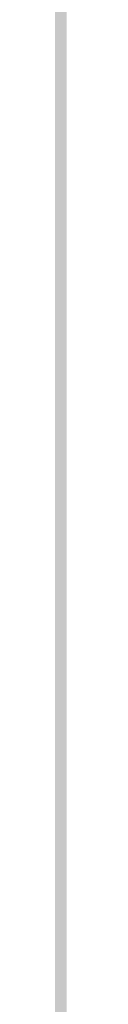
# Model space of a CAD drawing. Units: inches. Extents: x 2083 to 3317, y 1141 to 2115.
# Tile 209 of 256: x 3126.956 to 3126.958, y 1264.131 to 1265.165. Entities that reach past the tile are written whole.
import ezdxf

# ---------------------------------------------------------------- set-up
doc = ezdxf.new("R2010")
doc.units = ezdxf.units.IN
doc.layers.add('A-ANNO-DIMS', color=2, linetype='Continuous', lineweight=18)
doc.layers.add('A-WALL-PATT', color=251, linetype='Continuous', lineweight=13, true_color=0x636466)
doc.styles.get("Standard").update_dxf_attribs({"font": 'arial.ttf'})
doc.dimstyles.new('ISO-25', dxfattribs={"dimtxt": 12, "dimasz": 12, "dimexe": 1.25, "dimexo": 0.625, "dimtad": 1, "dimlunit": 3, "dimtxsty": 'Standard', "dimcen": 2.5, "dimadec": 0, "dimazin": 0, "dimtfac": 1, "dimtmove": 0, "dimatfit": 3, "dimfxl": 1, "dimarcsym": 0})

# ---------------------------------------------------------------- blocks, each defined once
blk = doc.blocks.new('*D26')
at = {"layer": 'A-ANNO-DIMS', "color": 0, "lineweight": -2, "transparency": 16777216}
for p, q in [((3088.9858, 1274.9151), (3088.9858, 1270.952)), ((3111.24, 1274.9151), (3111.24, 1270.952)), ((3076.9858, 1272.202), (2840.2624, 1272.202)), ((3111.24, 1272.202), (3088.9858, 1272.202)), ((3123.24, 1272.202), (3135.24, 1272.202))]:
    blk.add_line(p, q, dxfattribs=at)
at = {"layer": 'A-ANNO-DIMS', "color": 0, "transparency": 16777216}
for points in [[(3076.9858, 1274.202), (3076.9858, 1270.202), (3088.9858, 1272.202)], [(3123.24, 1274.202), (3123.24, 1270.202), (3111.24, 1272.202)]]:
    blk.add_solid(points, dxfattribs=at)
at = {"layer": 'Defpoints', "color": 0, "transparency": 16777216}
for p in [(3088.9858, 1275.5401), (3111.24, 1275.5401), (3088.9858, 1272.202)]:
    blk.add_point(p, dxfattribs=at)
at = {"layer": 'A-ANNO-DIMS', "color": 0, "transparency": 16777216, "insert": (2952.6241, 1279.0316), "char_height": 12, "attachment_point": 5}
blk.add_mtext('NIGHTSTAND 1\'-10 1/2" TYP.', dxfattribs=at)
blk = doc.blocks.new('*D27')
at = {"layer": 'A-ANNO-DIMS', "color": 0, "lineweight": -2, "transparency": 16777216}
for p, q in [((3114.5782, 1309.7943), (3114.5782, 1321.7943)), ((3111.865, 1297.7943), (3115.8282, 1297.7943)), ((3114.5782, 1297.7943), (3114.5782, 1275.5401)), ((3111.865, 1275.5401), (3115.8282, 1275.5401)), ((3114.5782, 1263.5401), (3114.5782, 1140.9886))]:
    blk.add_line(p, q, dxfattribs=at)
at = {"layer": 'A-ANNO-DIMS', "color": 0, "transparency": 16777216}
for points in [[(3112.5782, 1309.7943), (3116.5782, 1309.7943), (3114.5782, 1297.7943)], [(3112.5782, 1263.5401), (3116.5782, 1263.5401), (3114.5782, 1275.5401)]]:
    blk.add_solid(points, dxfattribs=at)
at = {"layer": 'Defpoints', "color": 0, "transparency": 16777216}
for p in [(3111.24, 1297.7943), (3111.24, 1275.5401), (3114.5782, 1275.5401)]:
    blk.add_point(p, dxfattribs=at)
at = {"layer": 'A-ANNO-DIMS', "color": 0, "transparency": 16777216, "insert": (3107.7485, 1196.2643), "char_height": 12, "attachment_point": 5, "rotation": 90}
blk.add_mtext('1\'-10 1/2" TYP.', dxfattribs=at)

msp = doc.modelspace()

# ---------------------------------------------------------------- hatches: boundary and pattern name
at = {"layer": 'A-WALL-PATT'}
h = msp.add_hatch(color=256, dxfattribs=at)
h.dxf.hatch_style = 1
h.paths.add_polyline_path([(3126.9598, 2020.7614), (2748.9598, 2020.7614), (2604.9598, 2020.7614), (2226.9598, 2020.7614), (2226.9598, 1702.7614), (2466.9598, 1702.7614), (2466.9598, 1582.7614), (2418.9598, 1582.7614), (2418.9598, 1477.7614), (2226.9598, 1477.7614), (2226.9598, 1263.2614), (2544.9598, 1263.2614), (2544.9598, 1411.7614), (2604.9598, 1411.7614), (2685.9598, 1411.7614), (2685.9598, 1420.7614), (2604.9598, 1420.7614), (2604.9598, 1573.7614), (2604.9598, 1702.7614), (2604.9598, 2011.7614), (2748.9598, 2011.7614), (2748.9598, 1702.7614), (2862.9598, 1702.7614), (2862.9598, 1621.7614), (2871.9598, 1621.7614), (2871.9598, 1702.7614), (2883.9598, 1702.7614), (2883.9598, 1706.9395, -0.026459), (2883.9598, 1711.7614), (2757.9598, 1711.7614), (2757.9598, 1807.7614), (2787.9598, 1807.7614), (2787.9598, 1812.2614), (2757.9598, 1812.2614), (2757.9598, 2011.7614), (2877.9598, 2011.7614), (2877.9598, 1812.2614), (2847.9598, 1812.2614), (2847.9598, 1807.7614), (2889.8357, 1807.7614), (2889.8357, 1812.2614), (2882.4598, 1812.2614), (2882.4598, 2011.7614), (3117.9598, 2011.7614), (3117.9598, 1812.2614), (2937.8357, 1812.2614), (2937.8357, 1807.7614), (2995.7098, 1807.7614), (2995.7098, 1796.1177), (3000.2098, 1796.1177), (3000.2098, 1807.7614), (3117.9598, 1807.7614), (3117.9598, 1711.7614), (3000.2098, 1711.7614), (3000.2098, 1760.1177), (2998.5727, 1760.1177, -0.020711), (2995.7098, 1760.1177), (2995.7098, 1711.7614), (2931.9598, 1711.7614), (2931.9598, 1702.7614), (3126.9598, 1702.7614)])
h.paths.add_polyline_path([(2471.4598, 2011.7614), (2471.4598, 1810.0114), (2462.7169, 1810.0114), (2462.7169, 1805.5114), (2505.9598, 1805.5114), (2505.9598, 1810.0114), (2475.9598, 1810.0114), (2475.9598, 2011.7614), (2595.9598, 2011.7614), (2595.9598, 1810.0114), (2565.9598, 1810.0114), (2565.9598, 1805.5114), (2595.9598, 1805.5114), (2595.9598, 1711.7614), (2235.9598, 1711.7614), (2235.9598, 1805.5114), (2353.7098, 1805.5114), (2353.7098, 1796.0542), (2358.2098, 1796.0542), (2358.2098, 1805.5114), (2414.7169, 1805.5114), (2414.7169, 1810.0114), (2235.9598, 1810.0114), (2235.9598, 2011.7614)], flags=16)
h.paths.add_polyline_path([(2270.2047, 1994.61), (2270.2047, 1970.61), (2246.2047, 1970.61), (2246.2047, 1994.61)], flags=0)
edge = h.paths.add_edge_path(flags=0)
edge.add_ellipse((2332.0274, 1899.7982), major_axis=(-3.043, 3.043), ratio=0.168252, start_angle=-161.3322, end_angle=-156.3071, ccw=False)
edge.add_ellipse((2333.082, 1898.7435), major_axis=(-1.0546, 1.0546), ratio=0.453532, start_angle=-123.371, end_angle=-94.1591)
edge = h.paths.add_edge_path(flags=0)
edge.add_ellipse((2332.0274, 1968.8763), major_axis=(3.043, 3.043), ratio=0.168252, start_angle=18.6678, end_angle=23.6929)
edge.add_spline(control_points=[(2332.9256, 1970.6911), (2332.2268, 1970.3361), (2330.8937, 1969.6589), (2328.4131, 1970.9321), (2327.2039, 1967.7487), (2324.7096, 1969.9556), (2322.5328, 1967.0124), (2320.0128, 1971.2958), (2317.6803, 1968.1578), (2316.0405, 1967.102), (2315.4269, 1966.8096)], knot_values=[0, 0, 0, 0, 2.267059, 4.324559, 6.685584, 8.878641, 11.121502, 14.300359, 17.755284, 19.732645, 19.732645, 19.732645, 19.732645], degree=3, periodic=0)
edge.add_ellipse((2332.0274, 1968.8763), major_axis=(3.043, 3.043), ratio=0.168252, start_angle=18.6678, end_angle=23.6929, ccw=False)
edge.add_ellipse((2333.082, 1969.9309), major_axis=(1.0546, 1.0546), ratio=0.453532, start_angle=56.629, end_angle=85.8409, ccw=False)
edge = h.paths.add_edge_path(flags=0)
edge.add_spline(control_points=[(2296.4283, 1967.9879), (2293.6278, 1965.3363), (2287.7036, 1959.7271), (2299.7439, 1949.9957), (2294.5326, 1935.6685), (2290.5732, 1920.6035), (2293.3941, 1909.9737), (2296.1854, 1904.9665)], knot_values=[0.099185, 0.099185, 0.099185, 0.099185, 0.345301, 0.619822, 0.982653, 1.386093, 1.810555, 1.810555, 1.810555, 1.810555], degree=3, periodic=0)
edge.add_spline(control_points=[(2296.1854, 1904.9665), (2297.3836, 1902.6193), (2298.001, 1901.9493), (2298.553, 1901.4682)], knot_values=[0.006246, 0.006246, 0.006246, 0.006246, 0.055476, 0.055476, 0.055476, 0.055476], degree=3, periodic=0)
edge.add_spline(control_points=[(2298.553, 1901.4682), (2297.2586, 1900.9232), (2295.2253, 1900.2321), (2293.0602, 1900.6142), (2292.1014, 1900.7884), (2292.0896, 1900.7906)], knot_values=[0.312835, 0.312835, 0.312835, 0.312835, 0.40178, 0.474987, 0.475903, 0.475903, 0.475903, 0.475903], degree=3, periodic=0)
edge.add_arc((2292.7936, 1904.6641), 3.937, 215.4209, 259.6982, ccw=False)
edge.add_spline(control_points=[(2289.5853, 1902.3823), (2289.4767, 1902.5351), (2289.3685, 1902.688), (2289.2609, 1902.8412)], knot_values=[0.102872, 0.102872, 0.102872, 0.102872, 0.116896, 0.116896, 0.116896, 0.116896], degree=3, periodic=0)
edge.add_spline(control_points=[(2289.2609, 1902.8412), (2288.6866, 1902.5502), (2287.64, 1902.0199), (2285.8813, 1901.874), (2283.853, 1901.5044), (2281.72, 1899.7105), (2278.467, 1899.4929), (2276.1571, 1901.8832), (2272.259, 1899.8041), (2267.7776, 1901.8432), (2262.2439, 1900.184), (2257.4149, 1901.7821), (2254.3184, 1900.7261), (2253.1783, 1900.3373)], knot_values=[0, 0, 0, 0, 1.907977, 3.477176, 5.261074, 7.972851, 11.680248, 13.717921, 16.939592, 22.789562, 27.502503, 33.595215, 37.145618, 37.145618, 37.145618, 37.145618], degree=3, periodic=0)
edge.add_line((2253.1783, 1900.3373), (2250.2442, 1902.8412))
edge.add_line((2250.2442, 1902.8412), (2250.2442, 1965.8333))
edge.add_line((2250.2442, 1965.8333), (2253.1783, 1968.3371))
edge.add_spline(control_points=[(2253.1783, 1968.3371), (2254.3184, 1967.9483), (2257.4149, 1966.8924), (2262.2439, 1968.4904), (2267.7776, 1966.8313), (2271.5267, 1968.5372), (2273.8759, 1967.8283), (2274.2067, 1967.7276)], knot_values=[0, 0, 0, 0, 0.09018, 0.244935, 0.364644, 0.513233, 0.537855, 0.537855, 0.537855, 0.537855], degree=3, periodic=0)
edge.add_arc((2274.3529, 1963.7933), 3.937, 72.0511, 92.1279, ccw=False)
edge.add_arc((2281.2969, 1985.23), 18.5963, 252.05113, 288.56572)
edge.add_arc((2292.3167, 1956.0289), 12.6461, 71.02679, 113.77822, ccw=False)
edge = h.paths.add_edge_path(flags=0)
edge.add_spline(control_points=[(2274.8994, 1951.8562), (2275.0662, 1951.6166), (2275.2327, 1951.3766), (2275.398, 1951.1359)], knot_values=[1.409916, 1.409916, 1.409916, 1.409916, 1.43159, 1.43159, 1.43159, 1.43159], degree=3, periodic=0)
edge.add_spline(control_points=[(2275.398, 1951.1359), (2275.7921, 1950.5619), (2276.1792, 1949.9838), (2276.5455, 1949.3971)], knot_values=[1.358238, 1.358238, 1.358238, 1.358238, 1.409916, 1.409916, 1.409916, 1.409916], degree=3, periodic=0)
edge.add_line((2276.5455, 1949.3971), (2277.4373, 1947.8622))
edge.add_spline(control_points=[(2277.4373, 1947.8622), (2276.3038, 1945.6731), (2274.6397, 1942.4269), (2274.6316, 1938.0939), (2272.7991, 1930.8515), (2274.3564, 1943.897), (2275.9477, 1947.9234), (2276.5455, 1949.3971)], knot_values=[0.005632, 0.005632, 0.005632, 0.005632, 0.186014, 0.266002, 0.357087, 0.59639, 0.739732, 0.739732, 0.739732, 0.739732], degree=3, periodic=0)
edge.add_spline(control_points=[(2276.5455, 1949.3971), (2276.1792, 1949.9838), (2275.7921, 1950.5619), (2275.398, 1951.1359)], knot_values=[1.358238, 1.358238, 1.358238, 1.358238, 1.409916, 1.409916, 1.409916, 1.409916], degree=3, periodic=0)
edge.add_spline(control_points=[(2275.398, 1951.1359), (2274.9425, 1950.0805), (2274.2078, 1948.0253), (2273.9346, 1944.8515), (2272.4685, 1937.6275), (2273.4662, 1945.6965), (2274.7006, 1951.0595), (2274.8994, 1951.8562)], knot_values=[0.104364, 0.104364, 0.104364, 0.104364, 0.189636, 0.269624, 0.36071, 0.600013, 0.644622, 0.644622, 0.644622, 0.644622], degree=3, periodic=0)
h.paths.add_polyline_path([(2269.1675, 1963.1276, -0.357527), (2268.1706, 1960.9764, -0.092561), (2268.1706, 1939.4363, -0.357527), (2269.1675, 1937.2851, -0.357527), (2267.0163, 1938.282, -0.164785), (2254.6856, 1938.282, -0.357527), (2252.5344, 1937.2851, -0.357527), (2253.5313, 1939.4363, -0.092561), (2253.5313, 1960.9764, -0.357527), (2252.5344, 1963.1276, -0.357527), (2254.6856, 1962.1307, -0.164785), (2267.0163, 1962.1307, -0.357527)], flags=0)
h.paths.add_polyline_path([(2248.8741, 1967.8018), (2248.8741, 1957.0277), (2249.4578, 1957.0277), (2249.4578, 1911.6468), (2248.8741, 1911.6468), (2248.8741, 1900.8727), (2246.5119, 1900.8727, 0.197327), (2244.1497, 1902.4569), (2244.1497, 1966.2176, 0.197327), (2246.5119, 1967.8018)], flags=0)
h.paths.add_polyline_path([(2269.1675, 1931.3893, -0.357527), (2268.1706, 1929.2381, -0.092561), (2268.1706, 1907.6981, -0.357527), (2269.1675, 1905.5469, -0.357527), (2267.0163, 1906.5438, -0.164785), (2254.6856, 1906.5438, -0.357527), (2252.5344, 1905.5469, -0.357527), (2253.5313, 1907.6981, -0.092561), (2253.5313, 1929.2381, -0.357527), (2252.5344, 1931.3893, -0.357527), (2254.6856, 1930.3925, -0.164785), (2267.0163, 1930.3925, -0.357527)], flags=0)
edge = h.paths.add_edge_path(flags=0)
edge.add_spline(control_points=[(2276.1969, 1906.7237), (2276.1681, 1909.0289), (2276.114, 1913.3719), (2270.5984, 1924.925), (2273.9052, 1919.0128), (2275.9217, 1916.2621), (2275.4746, 1912.4021), (2277.2579, 1910.3806), (2276.696, 1908.225), (2276.6462, 1906.813), (2276.6178, 1906.0084)], knot_values=[0, 0, 0, 0, 8.61026, 16.221274, 18.843057, 23.804898, 27.440828, 29.356102, 31.203478, 33.650687, 33.650687, 33.650687, 33.650687], degree=3, periodic=0)
edge.add_spline(control_points=[(2276.6178, 1906.0084), (2276.6233, 1905.6241), (2276.4977, 1904.6287), (2275.4418, 1903.8547), (2274.9373, 1903.0804), (2274.8591, 1902.8412)], knot_values=[0.156488, 0.156488, 0.156488, 0.156488, 0.184398, 0.231376, 0.250598, 0.250598, 0.250598, 0.250598], degree=3, periodic=0)
edge.add_line((2274.8591, 1902.8412), (2276.506, 1902.8412))
edge.add_spline(control_points=[(2276.506, 1902.8412), (2276.7883, 1903.0849), (2277.6651, 1904.1252), (2278.2495, 1904.3407), (2277.6539, 1908.5274), (2278.1557, 1906.2278), (2278.1005, 1905.2859), (2278.8467, 1904.069), (2277.8568, 1903.4149), (2277.8742, 1902.991), (2277.9036, 1902.8412)], knot_values=[0.059574, 0.059574, 0.059574, 0.059574, 0.080753, 0.103741, 0.16972, 0.176036, 0.207137, 0.240474, 0.262341, 0.27366, 0.27366, 0.27366, 0.27366], degree=3, periodic=0)
edge.add_line((2277.9036, 1902.8412), (2280.0298, 1902.8412))
edge.add_spline(control_points=[(2280.0298, 1902.8412), (2279.8882, 1903.0884), (2279.4993, 1903.9816), (2280.1523, 1905.9393), (2278.1036, 1909.6578), (2279.7624, 1907.1853), (2280.3279, 1904.8749), (2280.4851, 1903.4896), (2281.4633, 1903.2494), (2281.7583, 1902.9365), (2281.834, 1902.8412)], knot_values=[0.013856, 0.013856, 0.013856, 0.013856, 0.034874, 0.088867, 0.107879, 0.126738, 0.158714, 0.193757, 0.217487, 0.226722, 0.226722, 0.226722, 0.226722], degree=3, periodic=0)
edge.add_spline(control_points=[(2281.834, 1902.8412), (2281.7875, 1902.8267), (2281.647, 1902.783), (2281.3955, 1902.8595), (2281.0881, 1902.9852), (2280.7207, 1903.0609), (2280.3335, 1903.0257), (2280.1248, 1902.8989), (2280.0298, 1902.8412)], knot_values=[0, 0, 0, 0, 0.14413, 0.435517, 0.749276, 1.153046, 1.548371, 1.878348, 1.878348, 1.878348, 1.878348], degree=3, periodic=0)
edge.add_line((2280.0298, 1902.8412), (2277.9036, 1902.8412))
edge.add_spline(control_points=[(2277.9036, 1902.8412), (2277.8929, 1902.7959), (2277.8654, 1902.6796), (2277.6075, 1902.6875), (2277.2741, 1902.8007), (2276.8379, 1902.6198), (2276.5838, 1902.7893), (2276.506, 1902.8412)], knot_values=[0, 0, 0, 0, 0.127189, 0.326199, 0.628009, 1.24357, 1.515331, 1.515331, 1.515331, 1.515331], degree=3, periodic=0)
edge.add_line((2276.506, 1902.8412), (2274.8591, 1902.8412))
edge.add_spline(control_points=[(2274.8591, 1902.8412), (2274.8144, 1902.8986), (2274.7251, 1903.0134), (2274.4935, 1903.119), (2274.2443, 1902.9605), (2273.9371, 1903.1849), (2273.614, 1902.9831), (2273.4083, 1902.883), (2273.3223, 1902.8412)], knot_values=[0, 0, 0, 0, 0.21843, 0.436957, 0.687977, 0.990379, 1.398396, 1.69185, 1.69185, 1.69185, 1.69185], degree=3, periodic=0)
edge.add_spline(control_points=[(2273.3223, 1902.8412), (2273.6167, 1903.4457), (2274.274, 1904.5383), (2276.0272, 1904.5737), (2276.207, 1906.5836), (2276.1969, 1906.7237)], knot_values=[0.012227, 0.012227, 0.012227, 0.012227, 0.059472, 0.106218, 0.134458, 0.134458, 0.134458, 0.134458], degree=3, periodic=0)
h.paths.add_polyline_path([(2270.7761, 1897.7898), (2270.7761, 1873.7898), (2246.7761, 1873.7898), (2246.7761, 1897.7898)], flags=0)
h.paths.add_polyline_path([(2353.7098, 1760.0051), (2353.7098, 1760.0542), (2358.2098, 1760.0542, -0.033729)], flags=0)
h.paths.add_polyline_path([(2321.8191, 1737.5292), (2341.9953, 1737.5292, -0.414214), (2343.2033, 1736.3212), (2343.2033, 1721.0206, -0.414214), (2341.9953, 1719.8127), (2321.8191, 1719.8127, -0.414214), (2320.6112, 1721.0206), (2320.6112, 1736.3212, -0.414214)], flags=0)
h.paths.add_polyline_path([(2324.235, 1736.3212), (2339.5794, 1736.3212, -0.414214), (2341.9953, 1733.9053), (2341.9953, 1725.4497, -0.414214), (2339.5794, 1723.0338), (2333.6806, 1723.0338), (2333.8453, 1722.0455, -0.870646), (2335.4254, 1721.8259, -0.767327), (2333.9227, 1721.4232), (2331.291, 1721.4232, -0.767327), (2329.7883, 1721.8259, -0.870646), (2331.3684, 1722.0455), (2331.5331, 1723.0338), (2324.235, 1723.0338, -0.414214), (2321.8191, 1725.4497), (2321.8191, 1733.9053, -0.414214)], flags=0)
h.paths.add_polyline_path([(2570.4838, 1928.6154), (2589.6838, 1928.6154), (2590.1688, 1928.6154), (2590.1688, 1904.9934), (2570.4838, 1904.9934)], flags=0)
h.paths.add_polyline_path([(2574.4473, 1927.2638, -1), (2572.8288, 1927.2638, -1)], flags=0)
h.paths.add_polyline_path([(2573.0899, 1926.9409), (2573.925, 1927.776), (2574.1477, 1927.5533), (2573.3126, 1926.7182)], flags=0)
h.paths.add_polyline_path([(2578.7791, 1919.7296, -1), (2571.5917, 1919.7296, -1)], flags=0)
h.paths.add_polyline_path([(2578.3854, 1919.7296, -1), (2571.9854, 1919.7296, -1)], flags=0)
h.paths.add_polyline_path([(2331.5958, 1729.4762, -1), (2333.618, 1729.4762, -1)], flags=0)
h.paths.add_polyline_path([(2578.0342, 1927.2638, -1), (2576.4157, 1927.2638, -1)], flags=0)
h.paths.add_polyline_path([(2576.6889, 1927.5311), (2576.9116, 1927.7538), (2577.7467, 1926.9186), (2577.524, 1926.6959)], flags=0)
h.paths.add_polyline_path([(2578.1391, 1909.8595, -1), (2572.2317, 1909.8595, -1)], flags=0)
h.paths.add_polyline_path([(2577.7454, 1909.8595, -1), (2572.6254, 1909.8595, -1)], flags=0)
h.paths.add_polyline_path([(2583.7977, 1927.2638, -1), (2582.1792, 1927.2638, -1)], flags=0)
h.paths.add_polyline_path([(2582.7186, 1927.7538), (2583.5538, 1926.9186), (2583.3311, 1926.6959), (2582.4959, 1927.5311)], flags=0)
h.paths.add_polyline_path([(2582.4959, 1927.5311), (2582.7186, 1927.7538), (2583.5538, 1926.9186), (2583.3311, 1926.6959)], flags=0)
h.paths.add_polyline_path([(2587.7391, 1920.5296, -1), (2581.8317, 1920.5296, -1)], flags=0)
h.paths.add_polyline_path([(2587.3454, 1920.5296, -1), (2582.2254, 1920.5296, -1)], flags=0)
h.paths.add_polyline_path([(2587.3846, 1927.2638, -1), (2585.7661, 1927.2638, -1)], flags=0)
h.paths.add_polyline_path([(2586.082, 1926.9802), (2586.9172, 1927.8154), (2587.1399, 1927.5927), (2586.3047, 1926.7575)], flags=0)
h.paths.add_polyline_path([(2588.3791, 1910.6595, -1), (2581.1917, 1910.6595, -1)], flags=0)
h.paths.add_polyline_path([(2587.9854, 1910.6595, -1), (2581.5854, 1910.6595, -1)], flags=0)
h.paths.add_polyline_path([(2417.1677, 1729.4779), (2437.3439, 1729.4779, -0.414214), (2438.5519, 1728.2699), (2438.5519, 1712.9693, -0.414214), (2437.3439, 1711.7614), (2417.1677, 1711.7614, -0.414214), (2415.9598, 1712.9693), (2415.9598, 1728.2699, -0.414214)], flags=0)
h.paths.add_polyline_path([(2419.5836, 1728.2699), (2434.928, 1728.2699, -0.414214), (2437.3439, 1725.8541), (2437.3439, 1717.3984, -0.414214), (2434.928, 1714.9825), (2429.0292, 1714.9825), (2429.1939, 1713.9942, -0.870646), (2430.774, 1713.7746, -0.767327), (2429.2713, 1713.372), (2426.6396, 1713.372, -0.767327), (2425.1369, 1713.7746, -0.870646), (2426.717, 1713.9942), (2426.8817, 1714.9825), (2419.5836, 1714.9825, -0.414214), (2417.1677, 1717.3984), (2417.1677, 1725.8541, -0.414214)], flags=0)
h.paths.add_polyline_path([(2419.5836, 1728.2699), (2434.928, 1728.2699, -0.414214), (2437.3439, 1725.8541), (2437.3439, 1717.3984, -0.414214), (2434.928, 1714.9825), (2429.0292, 1714.9825), (2428.3581, 1719.009), (2427.5528, 1719.009), (2426.8817, 1714.9825), (2419.5836, 1714.9825, -0.414214), (2417.1677, 1717.3984), (2417.1677, 1725.8541, -0.414214)], flags=0)
h.paths.add_polyline_path([(2426.9444, 1721.4249, -1), (2428.9666, 1721.4249, -1)], flags=0)
h.paths.add_polyline_path([(2475.9598, 1702.7614), (2595.9598, 1702.7614), (2595.9598, 1582.7614), (2475.9598, 1582.7614)], flags=16)
h.paths.add_polyline_path([(2427.9598, 1573.7614), (2595.9598, 1573.7614), (2595.9598, 1468.7614), (2595.9598, 1420.7614), (2384.4598, 1420.7614), (2384.4598, 1468.7614), (2427.9598, 1468.7614)], flags=16)
h.paths.add_polyline_path([(2379.9598, 1468.7614), (2379.9598, 1420.7614), (2235.9598, 1420.7614), (2235.9598, 1468.7614)], flags=16)
h.paths.add_polyline_path([(2317.816, 1466.6958), (2337.9922, 1466.6958, -0.414214), (2339.2002, 1465.4878), (2339.2002, 1450.1872, -0.414214), (2337.9922, 1448.9792), (2317.816, 1448.9792, -0.414214), (2316.6081, 1450.1872), (2316.6081, 1465.4878, -0.414214)], flags=0)
h.paths.add_polyline_path([(2320.2319, 1465.4878), (2335.5763, 1465.4878, -0.414214), (2337.9922, 1463.0719), (2337.9922, 1454.6163, -0.414214), (2335.5763, 1452.2004), (2329.6775, 1452.2004), (2329.8422, 1451.212, -0.870646), (2331.4223, 1450.9925, -0.767327), (2329.9196, 1450.5898), (2327.2879, 1450.5898, -0.767327), (2325.7852, 1450.9925, -0.870646), (2327.3653, 1451.212), (2327.53, 1452.2004), (2320.2319, 1452.2004, -0.414214), (2317.816, 1454.6163), (2317.816, 1463.0719, -0.414214)], flags=0)
h.paths.add_polyline_path([(2320.2319, 1465.4878), (2335.5763, 1465.4878, -0.414214), (2337.9922, 1463.0719), (2337.9922, 1454.6163, -0.414214), (2335.5763, 1452.2004), (2329.6775, 1452.2004), (2329.0064, 1456.2269), (2328.2011, 1456.2269), (2327.53, 1452.2004), (2320.2319, 1452.2004, -0.414214), (2317.816, 1454.6163), (2317.816, 1463.0719, -0.414214)], flags=0)
h.paths.add_polyline_path([(2327.5926, 1458.6428, -1), (2329.6148, 1458.6428, -1)], flags=0)
h.paths.add_polyline_path([(2244.4117, 1433.3405), (2241.9209, 1433.3405, -0.414214), (2240.0179, 1435.2435), (2240.0179, 1440.9528, -0.414211), (2241.9209, 1442.8559), (2244.4117, 1442.8559, -1.976472)], flags=0)
h.paths.add_polyline_path([(2245.3569, 1434.3975, -0.414214), (2245.3569, 1441.7988, -2.144098)], flags=0)
h.paths.add_polyline_path([(2535.9598, 1416.2614), (2535.9598, 1272.2614), (2235.9598, 1272.2614), (2235.9598, 1416.2614)], flags=16)
h.paths.add_polyline_path([(2260.1196, 1384.2928), (2260.1196, 1362.0386), (2237.8654, 1362.0386), (2237.8654, 1384.2928)], flags=0)
edge = h.paths.add_edge_path(flags=0)
edge.add_line((2318.2518, 1362.0933), (2318.1458, 1362.001))
edge.add_ellipse((2317.4451, 1360.431), major_axis=(2.8216, 2.8216), ratio=0.168252, start_angle=18.6678, end_angle=20.9481, ccw=False)
edge.add_ellipse((2318.423, 1361.409), major_axis=(0.9779, 0.9779), ratio=0.453532, start_angle=56.629, end_angle=70.2262, ccw=False)
edge = h.paths.add_edge_path(flags=0)
edge.add_line((2319.1074, 1295.5711), (2319.015, 1295.6771))
edge.add_ellipse((2317.4451, 1296.3778), major_axis=(-2.8216, 2.8216), ratio=0.168252, start_angle=-161.3322, end_angle=-159.0519, ccw=False)
edge.add_ellipse((2318.423, 1295.3999), major_axis=(-0.9779, 0.9779), ratio=0.453532, start_angle=-123.371, end_angle=-109.7738)
edge = h.paths.add_edge_path(flags=0)
edge.add_spline(control_points=[(2284.2103, 1301.1702), (2284.5807, 1300.4447), (2284.8912, 1299.892), (2285.1596, 1299.461)], knot_values=[0.039066, 0.039066, 0.039066, 0.039066, 0.055476, 0.055476, 0.055476, 0.055476], degree=3, periodic=0)
edge.add_line((2285.1596, 1299.461), (2284.2103, 1301.1702))
edge = h.paths.add_edge_path(flags=0)
edge.add_line((2280.4125, 1297.298), (2283.37, 1297.0361))
edge.add_line((2283.37, 1297.0361), (2286.4057, 1297.9263))
edge.add_spline(control_points=[(2286.4057, 1297.9263), (2285.3055, 1297.4631), (2284.3448, 1297.1292), (2283.37, 1297.0361)], knot_values=[0.394369, 0.394369, 0.394369, 0.394369, 0.475903, 0.475903, 0.475903, 0.475903], degree=3, periodic=0)
edge.add_spline(control_points=[(2283.37, 1297.0361), (2283.2814, 1297.0277), (2282.3163, 1296.9573), (2281.3125, 1297.1345), (2280.4234, 1297.296), (2280.4125, 1297.298)], knot_values=[0.312835, 0.312835, 0.312835, 0.312835, 0.320246, 0.393453, 0.394369, 0.394369, 0.394369, 0.394369], degree=3, periodic=0)
edge = h.paths.add_edge_path(flags=0)
edge.add_line((2284.4356, 1359.6073), (2280.4463, 1355.328))
edge.add_line((2280.4463, 1355.328), (2279.58, 1351.0178))
edge.add_line((2279.58, 1351.0178), (2282.413, 1346.5804))
edge.add_spline(control_points=[(2282.413, 1346.5804), (2283.1533, 1345.5892), (2284.2529, 1344.0289), (2284.801, 1342.3872), (2284.9352, 1341.8055)], knot_values=[1.240098, 1.240098, 1.240098, 1.240098, 1.332892, 1.382712, 1.382712, 1.382712, 1.382712], degree=3, periodic=0)
edge.add_spline(control_points=[(2284.9352, 1341.8055), (2285.3191, 1340.1406), (2285.233, 1338.4092), (2284.9099, 1336.6541)], knot_values=[1.097484, 1.097484, 1.097484, 1.097484, 1.240098, 1.240098, 1.240098, 1.240098], degree=3, periodic=0)
edge.add_spline(control_points=[(2284.9099, 1336.6541), (2284.5868, 1334.899), (2284.0267, 1333.1203), (2283.4626, 1331.3606)], knot_values=[0.95487, 0.95487, 0.95487, 0.95487, 1.097484, 1.097484, 1.097484, 1.097484], degree=3, periodic=0)
edge.add_line((2283.4626, 1331.3606), (2281.8904, 1326.1534))
edge.add_line((2281.8904, 1326.1534), (2280.7563, 1321.0561))
edge.add_line((2280.7563, 1321.0561), (2280.2992, 1316.002))
edge.add_line((2280.2992, 1316.002), (2280.7159, 1310.9501))
edge.add_line((2280.7159, 1310.9501), (2282.0281, 1305.9721))
edge.add_line((2282.0281, 1305.9721), (2284.2103, 1301.1702))
edge.add_spline(control_points=[(2284.2103, 1301.1702), (2283.3407, 1302.7302), (2282.6119, 1304.3365), (2282.0281, 1305.9721)], knot_values=[0.099185, 0.099185, 0.099185, 0.099185, 0.241799, 0.241799, 0.241799, 0.241799], degree=3, periodic=0)
edge.add_spline(control_points=[(2282.0281, 1305.9721), (2281.4443, 1307.6078), (2281.0055, 1309.2728), (2280.7159, 1310.9501)], knot_values=[0.241799, 0.241799, 0.241799, 0.241799, 0.384413, 0.384413, 0.384413, 0.384413], degree=3, periodic=0)
edge.add_spline(control_points=[(2280.7159, 1310.9501), (2280.4332, 1312.5876), (2280.2894, 1314.277), (2280.2989, 1315.962), (2280.2992, 1316.002)], knot_values=[0.384413, 0.384413, 0.384413, 0.384413, 0.523647, 0.527028, 0.527028, 0.527028, 0.527028], degree=3, periodic=0)
edge.add_spline(control_points=[(2280.2992, 1316.002), (2280.3123, 1317.687), (2280.4779, 1319.3679), (2280.7563, 1321.0561)], knot_values=[0.527028, 0.527028, 0.527028, 0.527028, 0.669642, 0.669642, 0.669642, 0.669642], degree=3, periodic=0)
edge.add_spline(control_points=[(2280.7563, 1321.0561), (2281.0346, 1322.7443), (2281.4259, 1324.4396), (2281.8904, 1326.1534)], knot_values=[0.669642, 0.669642, 0.669642, 0.669642, 0.812256, 0.812256, 0.812256, 0.812256], degree=3, periodic=0)
edge.add_spline(control_points=[(2281.8904, 1326.1534), (2282.2644, 1327.5333), (2282.7879, 1329.2618), (2283.3528, 1331.0178), (2283.4626, 1331.3606)], knot_values=[0.812256, 0.812256, 0.812256, 0.812256, 0.927087, 0.95487, 0.95487, 0.95487, 0.95487], degree=3, periodic=0)
edge.add_line((2283.4626, 1331.3606), (2284.9099, 1336.6541))
edge.add_line((2284.9099, 1336.6541), (2284.9352, 1341.8055))
edge.add_line((2284.9352, 1341.8055), (2282.413, 1346.5804))
edge.add_spline(control_points=[(2282.413, 1346.5804), (2281.2751, 1348.1038), (2280.0784, 1349.5703), (2279.58, 1351.0178)], knot_values=[1.382712, 1.382712, 1.382712, 1.382712, 1.525326, 1.525326, 1.525326, 1.525326], degree=3, periodic=0)
edge.add_spline(control_points=[(2279.58, 1351.0178), (2279.4433, 1351.4147), (2279.1363, 1352.8569), (2279.7352, 1354.2904), (2280.4463, 1355.328)], knot_values=[1.525326, 1.525326, 1.525326, 1.525326, 1.564439, 1.667941, 1.667941, 1.667941, 1.667941], degree=3, periodic=0)
edge.add_spline(control_points=[(2280.4463, 1355.328), (2281.4261, 1356.7578), (2282.9308, 1358.1826), (2284.4356, 1359.6073)], knot_values=[1.667941, 1.667941, 1.667941, 1.667941, 1.810555, 1.810555, 1.810555, 1.810555], degree=3, periodic=0)
edge.add_arc((2280.6231, 1348.5182), 11.7262, 71.02679, 113.77822)
edge.add_arc((2270.4049, 1375.5952), 17.2436, 252.05113, 288.56572, ccw=False)
edge.add_arc((2263.966, 1355.7178), 3.6506, 72.0511, 92.1279)
edge.add_arc((2263.966, 1355.7178), 3.6506, 92.1279, 177.9851)
edge.add_spline(control_points=[(2260.3176, 1355.8462), (2260.2604, 1354.2207), (2260.5513, 1350.1865), (2262.9993, 1346.7663), (2264.4727, 1344.649)], knot_values=[1.43159, 1.43159, 1.43159, 1.43159, 1.564144, 1.770695, 1.770695, 1.770695, 1.770695], degree=3, periodic=0)
edge.add_line((2264.4727, 1344.649), (2264.9356, 1343.9825))
edge.add_spline(control_points=[(2263.801, 1340.2481), (2263.8432, 1340.5141), (2264.0672, 1341.7565), (2264.5127, 1343.0025), (2264.935, 1343.9811)], knot_values=[0.53657, 0.53657, 0.53657, 0.53657, 0.559349, 0.644622, 0.644622, 0.644622, 0.644622], degree=3, periodic=0)
edge.add_spline(control_points=[(2264.935, 1343.9811), (2265.1178, 1343.715), (2265.2989, 1343.4479), (2265.4768, 1343.1794)], knot_values=[1.384077, 1.384077, 1.384077, 1.384077, 1.409916, 1.409916, 1.409916, 1.409916], degree=3, periodic=0)
edge.add_spline(control_points=[(2265.4768, 1343.1794), (2265.6546, 1342.9108), (2265.8293, 1342.6408), (2265.9991, 1342.3688)], knot_values=[1.358238, 1.358238, 1.358238, 1.358238, 1.384077, 1.384077, 1.384077, 1.384077], degree=3, periodic=0)
edge.add_line((2265.9991, 1342.3688), (2266.826, 1340.9455))
edge.add_spline(control_points=[(2266.826, 1340.9455), (2268.8944, 1337.0897), (2271.3982, 1325.843), (2270.5162, 1310.5686), (2275.9194, 1301.8606), (2277.7895, 1299.1994)], knot_values=[0.116896, 0.116896, 0.116896, 0.116896, 0.472987, 1.050969, 1.313793, 1.313793, 1.313793, 1.313793], degree=3, periodic=0)
edge.add_spline(control_points=[(2277.7895, 1299.1994), (2277.8394, 1299.1285), (2277.8894, 1299.0575), (2277.9396, 1298.9866)], knot_values=[0.109884, 0.109884, 0.109884, 0.109884, 0.116896, 0.116896, 0.116896, 0.116896], degree=3, periodic=0)
edge.add_line((2277.9396, 1298.9866), (2277.7888, 1299.1991))
edge.add_spline(control_points=[(2277.7888, 1299.1991), (2277.2566, 1298.9294), (2276.2864, 1298.4379), (2275.0394, 1298.3344), (2274.3833, 1298.2389), (2274.2153, 1298.2093)], knot_values=[33.12187, 33.12187, 33.12187, 33.12187, 35.029056, 36.598255, 37.144827, 37.144827, 37.144827, 37.144827], degree=3, periodic=0)
edge.add_line((2274.2153, 1298.2093), (2273.0731, 1297.893))
edge.add_spline(control_points=[(2273.0731, 1297.893), (2272.3229, 1297.5798), (2271.0392, 1296.5105), (2269.2484, 1296.2261), (2268.4231, 1296.3747)], knot_values=[26.532584, 26.532584, 26.532584, 26.532584, 29.198919, 31.839101, 31.839101, 31.839101, 31.839101], degree=3, periodic=0)
edge.add_line((2268.4231, 1296.3747), (2263.8785, 1297.4575))
edge.add_spline(control_points=[(2263.8785, 1297.4575), (2263.5561, 1297.3594), (2261.8603, 1296.8387), (2260.2388, 1297.2824), (2258.9335, 1297.5165)], knot_values=[15.919551, 15.919551, 15.919551, 15.919551, 16.939592, 21.226067, 21.226067, 21.226067, 21.226067], degree=3, periodic=0)
edge.add_line((2258.9335, 1297.5165), (2254.0552, 1297.329))
edge.add_spline(control_points=[(2254.0552, 1297.329), (2253.7555, 1297.2958), (2252.1137, 1297.1652), (2250.4619, 1297.5442), (2249.1297, 1297.6679)], knot_values=[5.306517, 5.306517, 5.306517, 5.306517, 6.276435, 10.613034, 10.613034, 10.613034, 10.613034], degree=3, periodic=0)
edge.add_line((2249.1297, 1297.6679), (2244.3316, 1296.8778))
edge.add_line((2244.3316, 1296.8778), (2241.611, 1299.1994))
edge.add_line((2241.611, 1299.1994), (2241.611, 1357.6094))
edge.add_line((2241.611, 1357.6094), (2244.3316, 1359.9311))
edge.add_line((2244.3316, 1359.9311), (2252.7288, 1359.5427))
edge.add_spline(control_points=[(2252.7288, 1359.5427), (2252.8709, 1359.5464), (2253.3057, 1359.5482), (2253.7398, 1359.5143), (2254.0317, 1359.4824)], knot_values=[0.233291, 0.233291, 0.233291, 0.233291, 0.244935, 0.268927, 0.268927, 0.268927, 0.268927], degree=3, periodic=0)
edge.add_line((2254.0317, 1359.4824), (2259.5872, 1359.4164))
edge.add_spline(control_points=[(2259.5872, 1359.4164), (2260.6771, 1359.6285), (2262.0732, 1359.897), (2263.5237, 1359.4593), (2263.8304, 1359.366)], knot_values=[0.422516, 0.422516, 0.422516, 0.422516, 0.513233, 0.537855, 0.537855, 0.537855, 0.537855], degree=3, periodic=0)
edge.add_arc((2263.966, 1355.7178), 3.6506, 72.0511, 92.1279, ccw=False)
edge.add_arc((2270.4049, 1375.5952), 17.2436, 252.05113, 288.56572)
edge.add_arc((2280.6231, 1348.5182), 11.7262, 71.02679, 113.77822, ccw=False)
h.paths.add_polyline_path([(2240.3405, 1359.4347), (2240.3405, 1349.4444), (2240.8818, 1349.4444), (2240.8818, 1307.3645), (2240.3405, 1307.3645), (2240.3405, 1297.3741), (2238.1502, 1297.3741, 0.197327), (2235.9598, 1298.8431), (2235.9598, 1357.9657, 0.197327), (2238.1502, 1359.4347)], flags=0)
h.paths.add_polyline_path([(2259.1578, 1355.1005, -0.357527), (2258.2334, 1353.1058, -0.092561), (2258.2334, 1333.1326, -0.357527), (2259.1578, 1331.1379, -0.357527), (2257.1631, 1332.0622, -0.164785), (2245.7293, 1332.0622, -0.357527), (2243.7346, 1331.1379, -0.357527), (2244.6589, 1333.1326, -0.092561), (2244.6589, 1353.1058, -0.357527), (2243.7346, 1355.1005, -0.357527), (2245.7293, 1354.1761, -0.164785), (2257.1631, 1354.1761, -0.357527)], flags=0)
edge = h.paths.add_edge_path(flags=0)
edge.add_line((2265.9991, 1342.3688), (2266.826, 1340.9455))
edge.add_line((2266.826, 1340.9455), (2265.3076, 1337.8141))
edge.add_line((2265.3076, 1337.8141), (2264.3582, 1334.6529))
edge.add_line((2264.3582, 1334.6529), (2264.262, 1333.7997))
edge.add_spline(control_points=[(2264.262, 1333.7997), (2264.2084, 1333.1871), (2264.1621, 1332.3655), (2264.0071, 1331.4139), (2263.969, 1331.2018)], knot_values=[0.464444, 0.464444, 0.464444, 0.464444, 0.516691, 0.531608, 0.531608, 0.531608, 0.531608], degree=3, periodic=0)
edge.add_spline(control_points=[(2263.969, 1331.2018), (2263.7745, 1330.1189), (2263.4244, 1328.7908), (2263.2574, 1328.5307), (2263.234, 1328.5146)], knot_values=[0.372682, 0.372682, 0.372682, 0.372682, 0.44885, 0.464444, 0.464444, 0.464444, 0.464444], degree=3, periodic=0)
edge.add_spline(control_points=[(2263.234, 1328.5146), (2263.0964, 1328.4202), (2263.1312, 1329.3015), (2263.275, 1330.6157)], knot_values=[0.280919, 0.280919, 0.280919, 0.280919, 0.372682, 0.372682, 0.372682, 0.372682], degree=3, periodic=0)
edge.add_spline(control_points=[(2263.275, 1330.6157), (2263.4187, 1331.93), (2263.6715, 1333.6773), (2263.9699, 1335.315)], knot_values=[0.189157, 0.189157, 0.189157, 0.189157, 0.280919, 0.280919, 0.280919, 0.280919], degree=3, periodic=0)
edge.add_spline(control_points=[(2263.9699, 1335.315), (2264.1005, 1336.0322), (2264.4188, 1337.6219), (2264.7548, 1338.8644), (2264.9474, 1339.4911)], knot_values=[0.097394, 0.097394, 0.097394, 0.097394, 0.137578, 0.189157, 0.189157, 0.189157, 0.189157], degree=3, periodic=0)
edge.add_spline(control_points=[(2264.9474, 1339.4911), (2265.29, 1340.6061), (2265.6442, 1341.494), (2265.9991, 1342.3688)], knot_values=[0.005632, 0.005632, 0.005632, 0.005632, 0.097394, 0.097394, 0.097394, 0.097394], degree=3, periodic=0)
h.paths.add_polyline_path([(2259.1578, 1325.671, -0.357527), (2258.2334, 1323.6763, -0.092561), (2258.2334, 1303.7031, -0.357527), (2259.1578, 1301.7084, -0.357527), (2257.1631, 1302.6327, -0.164785), (2245.7293, 1302.6327, -0.357527), (2243.7346, 1301.7084, -0.357527), (2244.6589, 1303.7031, -0.092561), (2244.6589, 1323.6763, -0.357527), (2243.7346, 1325.671, -0.357527), (2245.7293, 1324.7466, -0.164785), (2257.1631, 1324.7466, -0.357527)], flags=0)
edge = h.paths.add_edge_path(flags=0)
edge.add_spline(control_points=[(2261.7089, 1317.3114), (2261.6795, 1317.4176), (2261.7619, 1317.3885), (2262.4907, 1316.0899), (2262.9622, 1315.3009)], knot_values=[14.955861, 14.955861, 14.955861, 14.955861, 16.221274, 18.694826, 18.694826, 18.694826, 18.694826], degree=3, periodic=0)
edge.add_spline(control_points=[(2262.9622, 1315.3009), (2262.9904, 1315.2536), (2263.7021, 1314.0674), (2264.349, 1313.1272), (2264.7301, 1312.1642)], knot_values=[18.694826, 18.694826, 18.694826, 18.694826, 18.843057, 22.433791, 22.433791, 22.433791, 22.433791], degree=3, periodic=0)
edge.add_spline(control_points=[(2264.7301, 1312.1642), (2264.8756, 1311.7964), (2265.1769, 1310.7698), (2265.1431, 1309.5593), (2265.2477, 1308.8242)], knot_values=[22.433791, 22.433791, 22.433791, 22.433791, 23.804898, 26.172756, 26.172756, 26.172756, 26.172756], degree=3, periodic=0)
edge.add_line((2265.2477, 1308.8242), (2265.8508, 1307.1719))
edge.add_spline(control_points=[(2265.8508, 1307.1719), (2266.065, 1306.8217), (2266.3844, 1306.3322), (2266.4244, 1305.7805), (2266.4204, 1305.6112)], knot_values=[28.062562, 28.062562, 28.062562, 28.062562, 29.356102, 29.911721, 29.911721, 29.911721, 29.911721], degree=3, periodic=0)
edge.add_spline(control_points=[(2266.4204, 1305.6112), (2266.4161, 1305.4326), (2266.394, 1305.25), (2266.3648, 1305.0659)], knot_values=[29.911721, 29.911721, 29.911721, 29.911721, 30.497837, 30.497837, 30.497837, 30.497837], degree=3, periodic=0)
edge.add_line((2266.3648, 1305.0659), (2266.0662, 1302.1363))
edge.add_spline(control_points=[(2266.0662, 1302.1363), (2266.0712, 1301.78), (2265.9981, 1301.2), (2265.6633, 1300.759), (2265.5089, 1300.5859)], knot_values=[0.156488, 0.156488, 0.156488, 0.156488, 0.184398, 0.203543, 0.203543, 0.203543, 0.203543], degree=3, periodic=0)
edge.add_line((2265.5089, 1300.5859), (2264.4353, 1299.1994))
edge.add_line((2264.4353, 1299.1994), (2265.9624, 1299.1994))
edge.add_line((2265.9624, 1299.1994), (2267.336, 1301.1753))
edge.add_line((2267.336, 1301.1753), (2267.3117, 1301.9862))
edge.add_spline(control_points=[(2267.3117, 1301.9862), (2267.2611, 1302.8624), (2267.1602, 1303.7371), (2267.2715, 1303.3259)], knot_values=[0.126229, 0.126229, 0.126229, 0.126229, 0.166617, 0.166617, 0.166617, 0.166617], degree=3, periodic=0)
edge.add_spline(control_points=[(2267.2715, 1303.3259), (2267.28, 1303.2943), (2267.3098, 1303.1754), (2267.3735, 1302.8836), (2267.4061, 1302.6828), (2267.4179, 1302.601)], knot_values=[0.166617, 0.166617, 0.166617, 0.166617, 0.16972, 0.176036, 0.180765, 0.180765, 0.180765, 0.180765], degree=3, periodic=0)
edge.add_spline(control_points=[(2267.7439, 1300.9875), (2267.6876, 1301.1509), (2267.4805, 1301.6567), (2267.4838, 1302.1448), (2267.4179, 1302.601)], knot_values=[0.180765, 0.180765, 0.180765, 0.180765, 0.193767, 0.220139, 0.220139, 0.220139, 0.220139], degree=3, periodic=0)
edge.add_line((2267.4179, 1302.601), (2267.7439, 1300.9875))
edge.add_spline(control_points=[(2267.7439, 1300.9875), (2267.832, 1300.7319), (2267.932, 1300.3099), (2267.5548, 1299.9745), (2267.4294, 1299.8292)], knot_values=[0.220139, 0.220139, 0.220139, 0.220139, 0.240474, 0.25489, 0.25489, 0.25489, 0.25489], degree=3, periodic=0)
edge.add_line((2267.4294, 1299.8292), (2267.2584, 1299.1994))
edge.add_line((2267.2584, 1299.1994), (2269.23, 1299.1994))
edge.add_spline(control_points=[(2269.23, 1299.1994), (2269.0987, 1299.4287), (2268.8428, 1300.0163), (2269.0116, 1300.9159), (2268.9468, 1301.6607)], knot_values=[0.013856, 0.013856, 0.013856, 0.013856, 0.034874, 0.067073, 0.067073, 0.067073, 0.067073], degree=3, periodic=0)
edge.add_line((2268.9468, 1301.6607), (2268.4316, 1303.6031))
edge.add_spline(control_points=[(2268.4316, 1303.6031), (2268.1756, 1304.1924), (2267.5962, 1305.2513), (2268.0407, 1304.6232), (2268.2514, 1304.2824)], knot_values=[0.090155, 0.090155, 0.090155, 0.090155, 0.107879, 0.120289, 0.120289, 0.120289, 0.120289], degree=3, periodic=0)
edge.add_spline(control_points=[(2268.2514, 1304.2824), (2268.3609, 1304.1053), (2269.0578, 1302.918), (2269.3827, 1301.5904), (2269.5214, 1300.7759), (2269.5752, 1300.5558)], knot_values=[0.120289, 0.120289, 0.120289, 0.120289, 0.126738, 0.158714, 0.173506, 0.173506, 0.173506, 0.173506], degree=3, periodic=0)
edge.add_line((2269.5752, 1300.5558), (2270.6858, 1299.4213))
edge.add_spline(control_points=[(2270.6858, 1299.4213), (2270.7672, 1299.3573), (2270.8379, 1299.2814), (2270.9029, 1299.1994)], knot_values=[0.21816, 0.21816, 0.21816, 0.21816, 0.226722, 0.226722, 0.226722, 0.226722], degree=3, periodic=0)
edge.add_line((2270.9372, 1299.1929), (2270.9029, 1299.1994))
edge.add_spline(control_points=[(2270.9029, 1299.1994), (2270.8598, 1299.186), (2270.7295, 1299.1455), (2270.4963, 1299.2164), (2270.2717, 1299.3083), (2270.121, 1299.348), (2270.0633, 1299.3596)], knot_values=[0.939174, 0.939174, 0.939174, 0.939174, 1.083304, 1.374691, 1.68845, 1.878348, 1.878348, 1.878348, 1.878348], degree=3, periodic=0)
edge.add_line((2270.0633, 1299.3596), (2269.23, 1299.1994))
edge.add_line((2269.23, 1299.1994), (2267.2584, 1299.1994))
edge.add_spline(control_points=[(2267.2584, 1299.1994), (2267.2484, 1299.1574), (2267.223, 1299.0497), (2266.9838, 1299.0569), (2266.8092, 1299.1162), (2266.6769, 1299.1091), (2266.6365, 1299.1048)], knot_values=[0.757665, 0.757665, 0.757665, 0.757665, 0.884854, 1.083864, 1.385675, 1.515331, 1.515331, 1.515331, 1.515331], degree=3, periodic=0)
edge.add_spline(control_points=[(2266.6365, 1299.1048), (2266.4852, 1299.0888), (2266.2358, 1299.0171), (2266.0346, 1299.1513), (2265.9624, 1299.1994)], knot_values=[0, 0, 0, 0, 0.485905, 0.757665, 0.757665, 0.757665, 0.757665], degree=3, periodic=0)
edge.add_line((2265.9624, 1299.1994), (2264.4353, 1299.1994))
edge.add_line((2264.4353, 1299.1994), (2263.8584, 1299.3671))
edge.add_spline(control_points=[(2263.8584, 1299.3671), (2263.8189, 1299.3709), (2263.7795, 1299.3857), (2263.7401, 1299.4015)], knot_values=[0.845925, 0.845925, 0.845925, 0.845925, 0.978627, 0.978627, 0.978627, 0.978627], degree=3, periodic=0)
edge.add_line((2263.7218, 1299.3964), (2263.0103, 1299.1994))
edge.add_spline(control_points=[(2263.0103, 1299.1994), (2263.2458, 1299.6829), (2263.506, 1300.1281), (2263.8735, 1300.408)], knot_values=[0.012227, 0.012227, 0.012227, 0.012227, 0.052971, 0.052971, 0.052971, 0.052971], degree=3, periodic=0)
edge.add_spline(control_points=[(2263.8735, 1300.408), (2263.9321, 1300.4527), (2264.0842, 1300.553), (2264.2552, 1300.6242), (2264.3597, 1300.6647)], knot_values=[0.052971, 0.052971, 0.052971, 0.052971, 0.059472, 0.069086, 0.069086, 0.069086, 0.069086], degree=3, periodic=0)
edge.add_line((2264.3597, 1300.6647), (2265.1419, 1301.0778))
edge.add_line((2265.1419, 1301.0778), (2265.6758, 1302.7996))
edge.add_line((2265.6758, 1302.7996), (2265.5407, 1305.7041))
edge.add_line((2265.5407, 1305.7041), (2264.8031, 1309.3277))
edge.add_line((2264.8031, 1309.3277), (2263.0405, 1314.0918))
edge.add_spline(control_points=[(2263.0405, 1314.0918), (2262.3836, 1315.6714), (2261.796, 1316.9977), (2261.7089, 1317.3114)], knot_values=[11.216896, 11.216896, 11.216896, 11.216896, 14.955861, 14.955861, 14.955861, 14.955861], degree=3, periodic=0)
h.paths.add_polyline_path([(2871.9598, 1416.2614), (2895.91, 1416.2614), (2895.91, 1420.7614), (2871.9598, 1420.7614), (2871.9598, 1501.7614), (2862.9598, 1501.7614), (2862.9598, 1420.7614), (2805.9598, 1420.7614), (2805.9598, 1411.7614), (2862.9598, 1411.7614), (2862.9598, 1263.2614), (3126.9598, 1263.2614), (3126.9598, 1411.7614), (3126.9598, 1486.7614), (2943.9598, 1486.7614), (2943.9598, 1477.7614), (2967.8603, 1477.7614), (2967.8603, 1420.7614), (2943.91, 1420.7614), (2943.91, 1416.2614), (3117.9598, 1416.2614), (3117.9598, 1420.7614), (2972.3603, 1420.7614), (2972.3603, 1477.7614), (3117.9598, 1477.7614), (3117.9598, 1420.7614), (3117.9598, 1272.2614), (2871.9598, 1272.2614)], flags=0)
h.paths.add_polyline_path([(2457.1256, 1485.9425), (2527.6027, 1485.9425), (2527.6027, 1537.6357), (2457.1256, 1537.6357)], flags=8)
h.paths.add_polyline_path([(2481.0051, 1609.9818), (2590.7658, 1609.9818), (2590.7658, 1682.0034), (2481.0051, 1682.0034)], flags=8)
h.paths.add_polyline_path([(2483.085, 1729.1268), (2553.562, 1729.1268), (2553.562, 1780.82), (2483.085, 1780.82)], flags=8)
h = msp.add_hatch(color=256, dxfattribs=at)
h.dxf.hatch_style = 1
h.paths.add_polyline_path([(3126.9598, 1486.7614), (2943.9598, 1486.7614), (2943.9598, 1477.7614), (2967.8603, 1477.7614), (2967.8603, 1420.7614), (2943.91, 1420.7614), (2943.91, 1416.2614), (3117.9598, 1416.2614), (3117.9598, 1420.7614), (2972.3603, 1420.7614), (2972.3603, 1477.7614), (3117.9598, 1477.7614), (3117.9598, 1420.7614), (3117.9598, 1272.2614), (2871.9598, 1272.2614), (2871.9598, 1416.2614), (2895.91, 1416.2614), (2895.91, 1420.7614), (2871.9598, 1420.7614), (2871.9598, 1501.7614), (2862.9598, 1501.7614), (2862.9598, 1420.7614), (2805.9598, 1420.7614), (2805.9598, 1411.7614), (2862.9598, 1411.7614), (2862.9598, 1263.2614), (3126.9598, 1263.2614), (3126.9598, 1411.7614)])

# ---------------------------------------------------------------- dimensions: what is measured, and where the dimension line sits
at = {"layer": 'A-ANNO-DIMS'}
for base, p1, p2, angle, text, picture, middle in [((3114.5782, 1275.5401), (3111.24, 1297.7943), (3111.24, 1275.5401), 270, '<> TYP.', '*D27', (3107.7485, 1196.2643)), ((3088.9858, 1272.202), (3111.24, 1275.5401), (3088.9858, 1275.5401), 180, 'NIGHTSTAND <> TYP.', '*D26', (2952.6241, 1279.0316))]:
    dim = msp.add_linear_dim(base=base, p1=p1, p2=p2, angle=angle, text=text, dimstyle='ISO-25', override={"dimdec": 1, "dimlfac": 1, "dimrnd": 0, "dimzin": 1, "dimdsep": 46, "dimlunit": 4, "dimfrac": 2}, dxfattribs=at)
    dim.commit()
    dim.dimension.update_dxf_attribs({"geometry": picture, "text_midpoint": middle})

doc.saveas('drawing.dxf')
